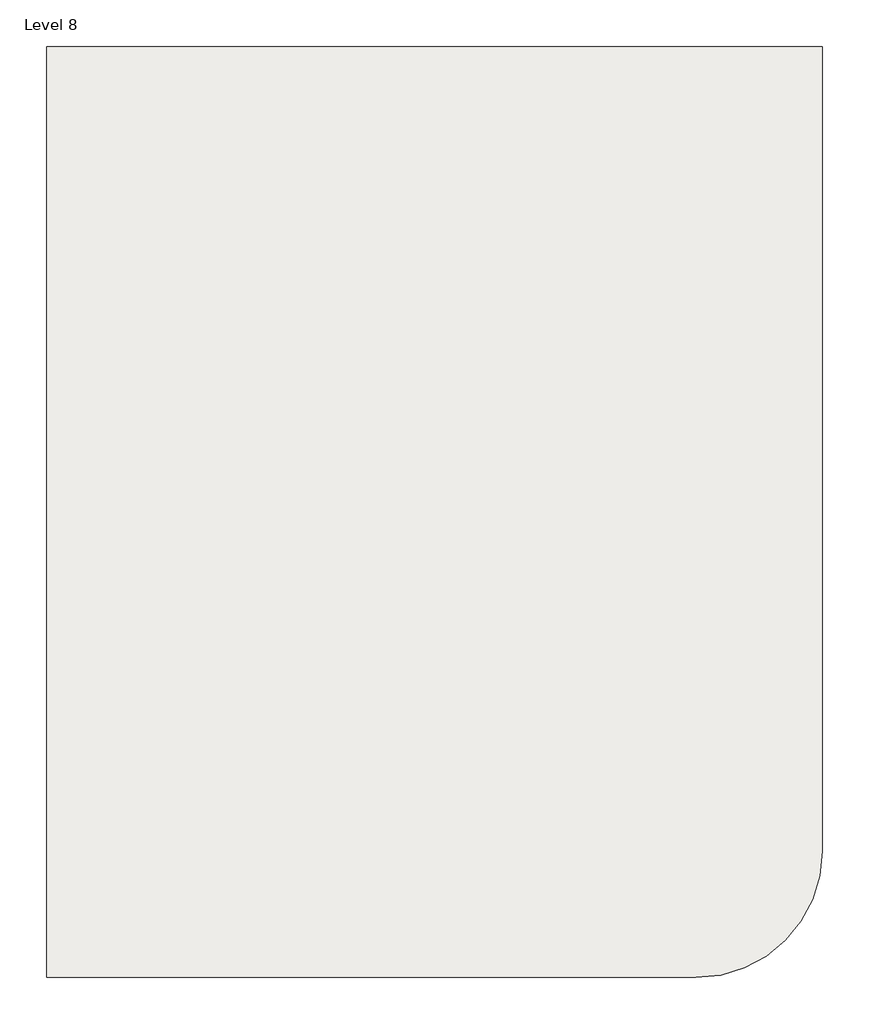
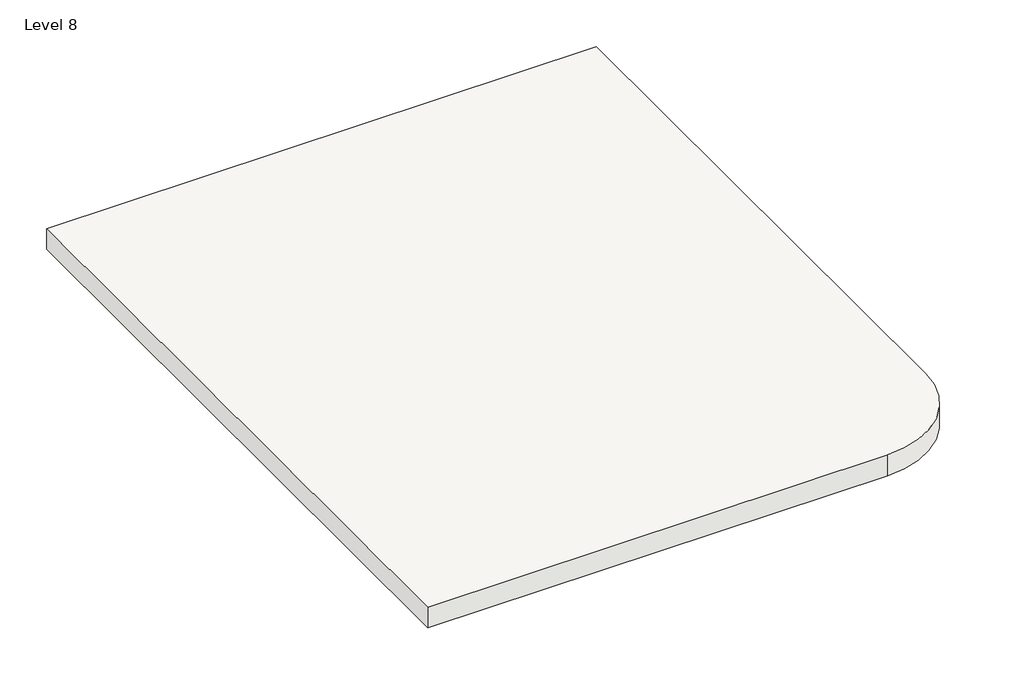
# One storey: 1 slab.
"""IFC4 building model written with IfcOpenShell, lengths in millimetres."""

from ifc_helpers import new_model, si_unit, point, frame, frame_2d, origin, place, context, project, spatial, polyline, circle_curve, trimmed, segment, composite_curve, outline, extrude, element, save

model = new_model("IFC4")

# Units and contexts
model_context = context("Model", 3, world=origin())
ifc_project = project(units=[si_unit("LENGTHUNIT", "METRE", prefix="MILLI")], contexts=[model_context])

# Site, building, storey
site = spatial("IfcSite", under=ifc_project)
building = spatial("IfcBuilding", under=site)
storey = spatial("IfcBuildingStorey", under=building, Name="Level 8", Elevation=21336.0)

# Slab
placement = place(None, origin())
element("IfcSlab", 1, ObjectType="Generic - 2' black 2", at=placement, inside=storey, context=model_context, shape_type="SweptSolid", body=[
    extrude(outline(composite_curve([segment(polyline([(6227.1926411, 14453.6432662), (6227.1926411, -1351.0107683)]), True, "CONTINUOUS"), segment(trimmed(circle_curve(frame_2d((3743.8466756, -1351.0107683)), 2483.3459655), [point((6227.1926411, -1351.0107683))], [point((3743.8466756, -3834.3567338))], False, "CARTESIAN"), True, "CONTINUOUS"), segment(polyline([(3743.8466756, -3834.3567338), (-9012.8073589, -3834.3567338), (-9012.8073589, 14453.6432662), (6227.1926411, 14453.6432662)]), True, "CONTINUOUS")], self_intersect=False)), frame((0.0, 0.0, 19812.0), z_axis=(0.0, 0.0, 1.0), x_axis=(1.0, 0.0, 0.0)), (0.0, 0.0, 1.0), 609.6),
])

save(model, "model.ifc")

# Revit data of these elements
# Type "Generic - 2' black 2"
#   Assembly Code = "B1010"
#   Function = 0
#   Layers, outside or top first: 2' - 0" "Door - Frame" (function 1)
# Element 1 (IfcSlab, "Generic - 2' black 2")
#   Height Offset From Level = -3' - 0"
#   Phase Created = New Construction
#   Materials on its faces: "Door - Frame"
# Materials
#   "Door - Frame": colour RGB 118 70 51, transparency 0, Cost = 0
